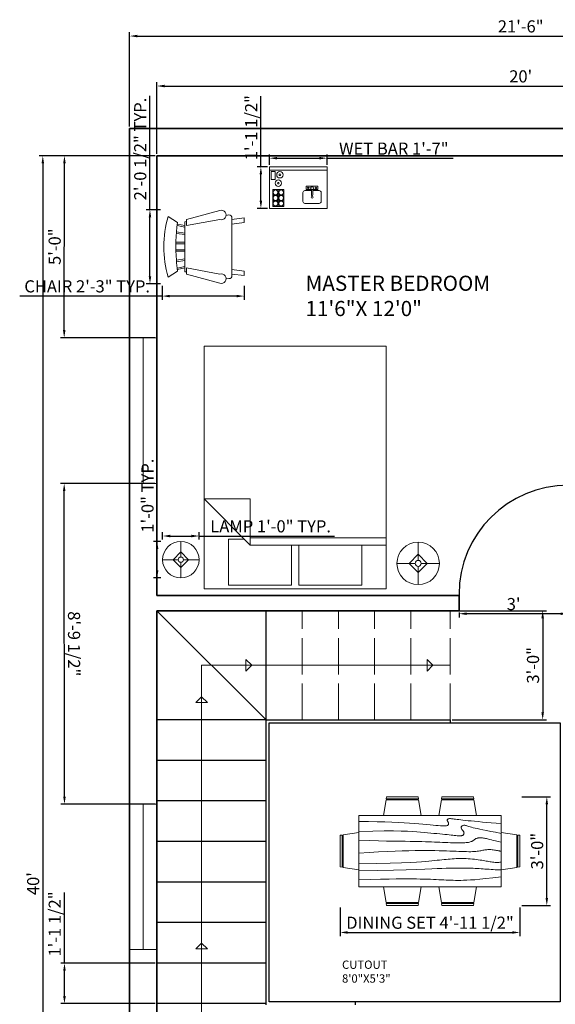
# Model space of a CAD drawing. Units: inches. Extents: x 2170 to 3011, y 1733 to 2338.
# Tile 2 of 5: x 2170 to 2347, y 2014 to 2338. Entities that reach past the tile are written whole.
import ezdxf

# ---------------------------------------------------------------- set-up
doc = ezdxf.new("R2010")
doc.units = ezdxf.units.IN
doc.linetypes.add('ACAD_ISO02W100', pattern=[15, 12, -3])
for name, color, linetype, lineweight in [('A-ANNO-SYMB', 2, 'Continuous', 13), ('A-AREA-IDEN', 4, 'Continuous', 18), ('A-FLOR-FIXT', 20, 'Continuous', 18), ('A-FLOR-OPEN', 7, 'Continuous', 25), ('A-FLOR-STRS-OVHD', 150, 'ACAD_ISO02W100', 18), ('A-WALL', 7, 'Continuous', 35), ('dim', 11, 'Continuous', 18), ('door', 6, 'Continuous', 25), ('furnitures', 20, 'Continuous', 18), ('stairs', 150, 'Continuous', 25), ('window', 3, 'Continuous', 20)]:
    doc.layers.add(name, color=color, linetype=linetype, lineweight=lineweight)
doc.styles.get("Standard").update_dxf_attribs({"font": 'arial.ttf'})
doc.dimstyles.new('ISO-25', dxfattribs={"dimtxt": 4, "dimasz": 2.5, "dimexe": 1.25, "dimexo": 0.625, "dimtad": 1, "dimlunit": 3, "dimtxsty": 'Standard', "dimcen": 2.5, "dimadec": 0, "dimazin": 0, "dimtfac": 1, "dimtmove": 0, "dimatfit": 3, "dimfxl": 1, "dimarcsym": 0})

# ---------------------------------------------------------------- blocks, each defined once
blk = doc.blocks.new('*U3')
for p, q in [((0, 0), (0, -6)), ((-40, 0), (-40, -6))]:
    blk.add_line(p, q)
blk.add_lwpolyline([(0, 0), (0, 40), (-1.75, 40), (-1.75, 0)], close=True)
blk.add_arc((0, 0), 40, 90, 180)
blk = doc.blocks.new('Bed - Queen')
for p, q in [((0, -80.00003), (0, 0)), ((0, 0), (59.99999, 0)), ((59.99999, 0), (59.99999, -80.00003)), ((7.99999, -1.2), (28.79998, -1.2)), ((7.99999, -14.4), (7.99999, -1.2)), ((28.79998, -1.2), (28.79998, -14.4)), ((31.19999, -1.2), (51.99999, -1.2)), ((31.19999, -14.4), (31.19999, -1.2)), ((51.99999, -1.2), (51.99999, -16.4)), ((0, -14.4), (44.8, -14.4)), ((59.99999, -29.6), (44.8, -14.4)), ((44.8, -14.4), (44.8, -29.6)), ((44.8, -16.8), (0, -16.8)), ((51.99999, -16.4), (46.79936, -16.4)), ((44.8, -29.6), (59.99999, -29.6)), ((59.99999, -80.00003), (0, -80.00003))]:
    blk.add_line(p, q)
blk = doc.blocks.new('Chair - Rocking')
for p, q in [((-8, -4.5), (-10, -1.5)), ((8, -4.5), (10, -1.5)), ((-7.5, -4.5), (-7, -7)), ((-6.5, -7), (-7.02225, -4.43)), ((-4.5, -7), (-4.96674, -4.19951)), ((-4, -7), (-4.40532, -4.16272)), ((-1.5, -4.05012), (-1.5, -7)), ((-1, -7), (-1, -4.05012)), ((1, -7), (1, -4.04655)), ((1.5, -4.05012), (1.5, -7)), ((4, -7), (4.40187, -4.18694)), ((4.5, -7), (4.96761, -4.19437)), ((6.5, -7), (7, -4.4057)), ((7.5, -4.5), (7, -7)), ((-9, -7.5), (-12, -18.49999)), ((-7, -7.5), (-9, -7.5)), ((-9, -18.49999), (-7, -7.5)), ((-8.23428, -6.99939), (-8.3093, -7.47958)), ((-8.23041, -7), (8.23915, -7)), ((7, -7.5), (9, -7.5)), ((9, -18.49999), (7, -7.5)), ((8.31071, -7.48854), (8.23449, -7.00073)), ((9, -7.5), (12, -18.49999)), ((-10.36644, -20.64523), (-10.5, -21.49999)), ((-9, -22.49999), (-9.5, -26.49999)), ((0, -22.49999), (-9.5, -22.49999)), ((-8, -26.49999), (-7.5, -22.49999)), ((0, -22.49999), (9.5, -22.49999)), ((8, -26.49999), (7.5, -22.49999)), ((9, -22.49999), (9.5, -26.49999)), ((10.5, -21.49999), (10.3575, -20.58798)), ((-9.5, -26.49999), (-8, -26.49999)), ((9.5, -26.49999), (8, -26.49999))]:
    blk.add_line(p, q)
for centre, radius, start, end in [((0, -34.08333), 34.08333, 72.93847, 107.0615), ((0, -68.25004), 64.25, 93.92211, 97.15267), ((0, -68.25004), 64.25, 82.84733, 93.92211), ((-10.5, -18.99999), 1.58114, 161.5651, 18.43495), ((10.5, -18.99999), 1.58114, 161.5651, 18.43495), ((-9.5, -21.49999), 1, 180, 270), ((9.5, -21.49999), 1, 270, 0)]:
    blk.add_arc(centre, radius, start, end)
blk = doc.blocks.new('Dining Set - 36 x 72 in.')
for p, q in [((-22.2343, 26.00059), (-23.4847, 17.99762)), ((-22.2304, 26), (-5.7608, 26)), ((-22, 27.5), (-22.1562, 26.50042)), ((-5.8416, 26.5), (-22.1534, 26.5)), ((-22, 27.5), (-6, 27.5)), ((-5.8437, 26.49966), (-6, 27.5)), ((-4.5152, 17.99762), (-5.7655, 25.99926)), ((5.7657, 26.00059), (4.5153, 17.99762)), ((5.7696, 26), (22.2392, 26)), ((6, 27.5), (5.8438, 26.50042)), ((22.1584, 26.5), (5.8466, 26.5)), ((6, 27.5), (22, 27.5)), ((22.1563, 26.49966), (22, 27.5)), ((23.4848, 17.99762), (22.2345, 25.99926)), ((36, 18), (-36, 18)), ((-36, 18), (-36, -18)), ((36, -18), (36, 18)), ((-45.5, 8), (-44.5004, 8.15617)), ((-45.5, 8), (-45.5, -8)), ((-44.5, -8.15843), (-44.5, 8.15338)), ((-44.0006, 8.23428), (-35.9976, 9.48474)), ((-44, 8.23041), (-44, -8.23915)), ((44.0006, 8.23428), (35.9976, 9.48474)), ((44, 8.23041), (44, -8.23915)), ((44.5, -8.15843), (44.5, 8.15338)), ((45.5, 8), (44.5005, 8.15617)), ((45.5, 8), (45.5, -8)), ((-44.4997, -8.15631), (-45.5, -8)), ((-35.9976, -9.48476), (-43.9993, -8.2345)), ((35.9976, -9.48476), (43.9993, -8.2345)), ((44.4997, -8.15631), (45.5, -8)), ((-36, -18), (36, -18)), ((-22.2343, -26.0006), (-23.4847, -17.99762)), ((-4.5152, -17.99762), (-5.7655, -25.99928)), ((5.7657, -26.0006), (4.5153, -17.99762)), ((23.4848, -17.99762), (22.2345, -25.99928)), ((-22.2304, -26), (-5.7608, -26)), ((-22, -27.5), (-22.1562, -26.50044)), ((-5.8416, -26.5), (-22.1534, -26.5)), ((-22, -27.5), (-6, -27.5)), ((-5.8437, -26.49967), (-6, -27.5)), ((5.7696, -26), (22.2392, -26)), ((6, -27.5), (5.8438, -26.50044)), ((22.1584, -26.5), (5.8466, -26.5)), ((6, -27.5), (22, -27.5)), ((22.1563, -26.49967), (22, -27.5))]:
    blk.add_line(p, q)
for points in [[(-36, 15), (-31.1772, 14.97754), (-26.8079, 14.91406), (-22.8538, 14.81543), (-19.276, 14.6875), (-16.0362, 14.53613), (-13.0957, 14.36718), (-10.4159, 14.18652), (-7.9583, 14), (-5.6904, 13.81315), (-3.6035, 13.63021), (-1.6954, 13.45508), (0.0365, 13.29166), (1.5945, 13.14388), (2.9811, 13.01562), (4.1988, 12.9108), (5.25, 12.83333), (6.1393, 12.78613), (6.8802, 12.76823), (7.4883, 12.77767), (7.9792, 12.8125), (8.3685, 12.87077), (8.6719, 12.95052), (8.9049, 13.0498), (9.0833, 13.16666), (9.2205, 13.29899), (9.3216, 13.44401), (9.3895, 13.59879), (9.4271, 13.76041), (9.4373, 13.92594), (9.4232, 14.09245), (9.3875, 14.257), (9.3333, 14.41666), (9.2638, 14.56917), (9.1836, 14.71484), (9.0975, 14.85465), (9.0104, 14.98958), (8.9272, 15.1206), (8.8529, 15.2487), (8.7922, 15.37483), (8.75, 15.5), (8.7305, 15.62467), (8.7344, 15.74739), (8.7617, 15.86621), (8.8125, 15.97916), (8.8867, 16.08431), (8.9844, 16.17968), (9.1055, 16.26334), (9.25, 16.33333), (9.4189, 16.38802), (9.6172, 16.42708), (9.8506, 16.45052), (10.125, 16.45833), (10.4463, 16.45052), (10.8203, 16.42708), (11.2529, 16.38802), (11.75, 16.33333), (12.3184, 16.26318), (12.9694, 16.17838), (13.7151, 16.07991), (14.5677, 15.96875), (15.5395, 15.84586), (16.6426, 15.71224), (17.8893, 15.56884), (19.2917, 15.41666), (20.859, 15.25667), (22.5879, 15.08984), (24.4721, 14.91715), (26.5052, 14.73958), (28.6809, 14.5581), (30.9929, 14.3737), (33.4347, 14.18733), (36, 14)], [(-36, 10), (-28.9766, 10.14274), (-23.1725, 10.20442), (-18.4241, 10.19775), (-14.5677, 10.13541), (-11.4399, 10.03011), (-8.877, 9.89453), (-6.7154, 9.74137), (-4.7917, 9.58333), (-2.9698, 9.43082), (-1.2246, 9.28515), (0.4415, 9.14534), (2.026, 9.01041), (3.5266, 8.87939), (4.9408, 8.7513), (6.266, 8.62516), (7.5, 8.5), (8.6411, 8.37549), (9.6914, 8.2539), (10.6538, 8.13818), (11.5312, 8.03125), (12.3267, 7.93603), (13.043, 7.85547), (13.6831, 7.79248), (14.25, 7.75), (14.7471, 7.7303), (15.1797, 7.73307), (15.5537, 7.75732), (15.875, 7.80208), (16.1494, 7.86637), (16.3828, 7.94922), (16.5811, 8.04964), (16.75, 8.16666), (16.8944, 8.29915), (17.0143, 8.44531), (17.1089, 8.60319), (17.1771, 8.77083), (17.218, 8.94629), (17.2305, 9.1276), (17.2137, 9.31282), (17.1667, 9.5), (17.0895, 9.6875), (16.987, 9.875), (16.8649, 10.0625), (16.7292, 10.25), (16.5856, 10.4375), (16.4401, 10.625), (16.2985, 10.8125), (16.1667, 11), (16.05, 11.18733), (15.9518, 11.3737), (15.8752, 11.5581), (15.8229, 11.73958), (15.798, 11.91715), (15.8034, 12.08984), (15.842, 12.25667), (15.9167, 12.41666), (16.0295, 12.56836), (16.1784, 12.70833), (16.3605, 12.83268), (16.5729, 12.9375), (16.8127, 13.01888), (17.0768, 13.07291), (17.3625, 13.0957), (17.6667, 13.08333), (17.9894, 13.03312), (18.3418, 12.94726), (18.7382, 12.82918), (19.1927, 12.68229), (19.7195, 12.51001), (20.3327, 12.31575), (21.0465, 12.10294), (21.875, 11.875), (22.8357, 11.63354), (23.959, 11.37304), (25.2786, 11.08618), (26.8282, 10.76562), (28.6414, 10.40405), (30.752, 9.99414), (33.1936, 9.52856), (36, 9)], [(-36, 5.5), (-30.7157, 5.3348), (-26.069, 5.20963), (-21.9946, 5.11767), (-18.4271, 5.05208), (-15.3009, 5.00602), (-12.5508, 4.97265), (-10.1112, 4.94515), (-7.9167, 4.91666), (-5.909, 4.88167), (-4.0586, 4.83984), (-2.3429, 4.79215), (-0.7396, 4.73958), (0.7739, 4.6831), (2.22, 4.6237), (3.6213, 4.56233), (5, 4.5), (6.373, 4.43782), (7.7344, 4.3776), (9.0723, 4.32129), (10.375, 4.27083), (11.6309, 4.22819), (12.8281, 4.19531), (13.9551, 4.17415), (15, 4.16666), (15.954, 4.17448), (16.819, 4.19791), (17.6001, 4.23698), (18.3021, 4.29166), (18.9299, 4.36198), (19.4883, 4.44791), (19.9823, 4.54948), (20.4167, 4.66666), (20.7969, 4.79899), (21.1302, 4.94401), (21.4245, 5.09879), (21.6875, 5.26041), (21.9271, 5.42594), (22.1511, 5.59245), (22.3672, 5.757), (22.5834, 5.91666), (22.8065, 6.06868), (23.0404, 6.21093), (23.2879, 6.34147), (23.5521, 6.45833), (23.8358, 6.55957), (24.142, 6.64323), (24.4735, 6.70735), (24.8334, 6.75), (25.2235, 6.76969), (25.642, 6.76692), (26.0858, 6.74267), (26.5521, 6.69791), (27.0379, 6.63362), (27.5404, 6.55078), (28.0565, 6.45036), (28.5834, 6.33333), (29.1242, 6.19987), (29.7071, 6.04687), (30.3661, 5.87044), (31.1354, 5.66666), (32.0493, 5.43164), (33.142, 5.16146), (34.4475, 4.85221), (36, 4.5)], [(-36, -1), (-30.7915, -0.6591), (-26.0195, -0.38216), (-21.6519, -0.16284), (-17.6563, 0.00521), (-14.0005, 0.12833), (-10.6523, 0.21289), (-7.5796, 0.26522), (-4.75, 0.29166), (-2.134, 0.29793), (0.2878, 0.28711), (2.5317, 0.26163), (4.6146, 0.22396), (6.5529, 0.17651), (8.3633, 0.12174), (10.0623, 0.06209), (11.6667, 0), (13.1899, -0.06201), (14.6341, -0.1211), (15.9982, -0.17432), (17.2813, -0.21875), (18.4823, -0.25147), (19.6003, -0.26953), (20.6343, -0.27002), (21.5834, -0.25), (22.4481, -0.20768), (23.2357, -0.14584), (23.9549, -0.06836), (24.6146, 0.02083), (25.2235, 0.11784), (25.7904, 0.21875), (26.3241, 0.31966), (26.8334, 0.41666), (27.3265, 0.50618), (27.8099, 0.58593), (28.2894, 0.65397), (28.7709, 0.70833), (29.2601, 0.74707), (29.763, 0.76823), (30.2855, 0.76985), (30.8334, 0.75), (31.4088, 0.70784), (31.9994, 0.64713), (32.589, 0.57275), (33.1615, 0.48958), (33.7008, 0.4025), (34.1908, 0.3164), (34.6153, 0.23616), (34.9584, 0.16666), (35.2099, 0.11165), (35.3848, 0.07031), (35.504, 0.04069), (35.5886, 0.02083), (35.6594, 0.00879), (35.7377, 0.0026), (35.8442, 0.00032), (36, 0)], [(-36, -6.5), (-27.1843, -6.31267), (-20.084, -6.1263), (-14.469, -5.9419), (-10.1094, -5.76042), (-6.7752, -5.58285), (-4.2363, -5.41016), (-2.2629, -5.24333), (-0.625, -5.08334), (0.8708, -4.93099), (2.2715, -4.78646), (3.5872, -4.64974), (4.8281, -4.52084), (6.0046, -4.39974), (7.127, -4.28646), (8.2053, -4.18099), (9.25, -4.08334), (10.2705, -3.99382), (11.2734, -3.91407), (12.2647, -3.84603), (13.25, -3.79167), (14.2354, -3.75293), (15.2266, -3.73177), (16.2295, -3.73015), (17.25, -3.75), (18.2912, -3.79248), (19.3451, -3.85547), (20.4009, -3.93604), (21.4479, -4.03125), (22.4754, -4.13819), (23.4727, -4.25391), (24.4289, -4.37549), (25.3334, -4.5), (26.1785, -4.62492), (26.9694, -4.74935), (27.7145, -4.87281), (28.4219, -4.99479), (29.1, -5.11483), (29.7572, -5.23242), (30.4016, -5.34709), (31.0417, -5.45834), (31.6837, -5.56437), (32.3262, -5.65821), (32.9658, -5.73153), (33.599, -5.77604), (34.2224, -5.78345), (34.8327, -5.74545), (35.4264, -5.65373), (36, -5.5)], [(-36, -10), (-26.4022, -9.81299), (-18.4675, -9.62891), (-11.9839, -9.45069), (-6.7396, -9.28125), (-2.5226, -9.12354), (0.8789, -8.98047), (3.6769, -8.85498), (6.0833, -8.75), (8.2767, -8.66765), (10.3021, -8.60677), (12.1712, -8.56543), (13.8958, -8.54167), (15.4876, -8.53353), (16.9583, -8.53907), (18.3197, -8.55632), (19.5834, -8.58334), (20.7616, -8.61841), (21.8685, -8.66081), (22.9188, -8.71004), (23.9271, -8.76563), (24.9081, -8.82707), (25.8763, -8.89388), (26.8465, -8.96558), (27.8334, -9.04167), (28.8474, -9.12118), (29.8828, -9.20117), (30.93, -9.27824), (31.9792, -9.34896), (33.0205, -9.40991), (34.0443, -9.45768), (35.0407, -9.48885), (36, -9.5)], [(-36, -14.5), (-30.0881, -14.33513), (-25.0332, -14.21224), (-20.7312, -14.12647), (-17.0781, -14.07292), (-13.97, -14.04671), (-11.3027, -14.04297), (-8.9724, -14.05681), (-6.875, -14.08334), (-4.9224, -14.11833), (-3.0905, -14.16016), (-1.3709, -14.20785), (0.2448, -14.26042), (1.7647, -14.3169), (3.1973, -14.3763), (4.5507, -14.43767), (5.8333, -14.5), (7.0554, -14.5621), (8.235, -14.62175), (9.3922, -14.67652), (10.5469, -14.72396), (11.7192, -14.76164), (12.929, -14.78711), (14.1965, -14.79794), (15.5417, -14.79167), (16.9933, -14.76424), (18.6152, -14.70508), (20.4804, -14.60197), (22.6615, -14.44271), (25.2312, -14.21509), (28.2624, -13.9069), (31.8277, -13.50594), (36, -13)]]:
    blk.add_lwpolyline(points)
blk = doc.blocks.new('Wet Bar')
for p, q in [((0, 0), (36, 0)), ((0, -26), (0, 0)), ((36, 0), (36, -26)), ((0, -2), (36, -2)), ((3.5, -3), (1, -3)), ((1, -3), (1, -8)), ((3.5, -8), (3.5, -3)), ((1, -8), (3.5, -8)), ((2, -14.25), (9, -14.25)), ((2, -24.75), (2, -14.25)), ((2, -17.75), (9, -17.75)), ((5.5, -14.25), (5.5, -24.75)), ((9, -14.25), (9, -24.75)), ((26.2, -17.55), (26.2, -14.1284)), ((27.1001, -17.55), (27.1001, -14.1284)), ((9, -21.25), (2, -21.25)), ((36, -26), (0, -26)), ((9, -24.75), (2, -24.75))]:
    blk.add_line(p, q)
for points in [[(26.2, -14.25), (22.95, -14.25), (22.95, -12.2), (26.75, -12.2)], [(26.7487, -12.2), (30.3501, -12.2), (30.3501, -14.25), (27.1001, -14.25)], [(20.95, -21.75), (20.95, -16.05)], [(22.15, -14.85), (26.2, -14.85)], [(27.1001, -14.85), (31.15, -14.85)], [(32.3501, -16.05), (32.3501, -21.75)], [(31.15, -22.95), (22.15, -22.95)]]:
    blk.add_lwpolyline(points)
for centre, radius in [((6.5, -5), 2), ((6.5, -5), 0.5), ((5.5, -10.25), 2), ((5.5, -10.25), 0.5), ((3.75, -16), 1.5), ((3.75, -19.5), 1.5), ((7.25, -16), 1.5), ((7.25, -19.5), 1.5), ((24.25, -13.25), 0.5), ((26.65, -13.35), 0.9), ((26.65, -19.05), 0.6), ((29, -13.25), 0.5), ((3.75, -23), 1.5), ((7.25, -23), 1.5)]:
    blk.add_circle(centre, radius)
for centre, radius, start, end in [((22.2251, -16.125), 1.2772, 93.36646, 176.6335), ((26.65, -17.55), 0.45, 180, 0), ((31.075, -16.125), 1.2772, 3.366461, 86.63354), ((22.2251, -21.675), 1.2772, 183.3665, 266.6335), ((31.075, -21.675), 1.2772, 273.3665, 356.6335)]:
    blk.add_arc(centre, radius, start, end)
blk = doc.blocks.new('Lamp - Table')
for p, q in [((0, 7), (0, 1)), ((-1, 0), (-7, 0)), ((0, 3), (-3, 0)), ((-3, 0), (0, -3)), ((3, 0), (0, 3)), ((0, -3), (3, 0)), ((1, 0), (7, 0)), ((0, -1), (0, -7))]:
    blk.add_line(p, q)
for radius in [7, 1]:
    blk.add_circle((0, 0), radius)
blk = doc.blocks.new('*D22')
at = {"layer": 'Defpoints', "color": 0, "transparency": 16777216}
for p in [(2455.17, 2316.33), (2215.17, 2293.31), (2455.17, 2293.31)]:
    blk.add_point(p, dxfattribs=at)
at = {"layer": 'dim', "color": 0, "lineweight": -2, "transparency": 16777216}
for p, q in [((2215.17, 2293.93), (2215.17, 2317.58)), ((2217.67, 2316.33), (2452.67, 2316.33)), ((2455.17, 2293.93), (2455.17, 2317.58))]:
    blk.add_line(p, q, dxfattribs=at)
at = {"layer": 'dim', "color": 0, "transparency": 16777216}
for points in [[(2217.67, 2316.74), (2217.67, 2315.91), (2215.17, 2316.33)], [(2452.67, 2316.74), (2452.67, 2315.91), (2455.17, 2316.33)]]:
    blk.add_solid(points, dxfattribs=at)
at = {"layer": 'dim', "color": 0, "transparency": 16777216, "insert": (2335.17, 2318.99), "char_height": 4, "attachment_point": 5}
blk.add_mtext("20'", dxfattribs=at)
blk = doc.blocks.new('*D23')
at = {"layer": 'Defpoints', "color": 0, "transparency": 16777216}
for p in [(2215.17, 2293.31), (2177.52, 1813.31), (2215.17, 1813.31)]:
    blk.add_point(p, dxfattribs=at)
at = {"layer": 'dim', "color": 0, "lineweight": -2, "transparency": 16777216}
for p, q in [((2214.54, 2293.31), (2176.27, 2293.31)), ((2177.52, 2290.81), (2177.52, 1815.81)), ((2214.54, 1813.31), (2176.27, 1813.31))]:
    blk.add_line(p, q, dxfattribs=at)
at = {"layer": 'dim', "color": 0, "transparency": 16777216}
for points in [[(2177.11, 2290.81), (2177.94, 2290.81), (2177.52, 2293.31)], [(2177.11, 1815.81), (2177.94, 1815.81), (2177.52, 1813.31)]]:
    blk.add_solid(points, dxfattribs=at)
at = {"layer": 'dim', "color": 0, "transparency": 16777216, "insert": (2174.86, 2053.31), "char_height": 4, "attachment_point": 5, "rotation": 90}
blk.add_mtext("40'", dxfattribs=at)
blk = doc.blocks.new('*D24')
at = {"layer": 'Defpoints', "color": 0, "transparency": 16777216}
for p in [(2314.84, 2143.31), (2350.84, 2143.31), (2314.84, 2142.31)]:
    blk.add_point(p, dxfattribs=at)
at = {"layer": 'dim', "color": 0, "lineweight": -2, "transparency": 16777216}
for p, q in [((2314.84, 2142.68), (2314.84, 2141.06)), ((2348.34, 2142.31), (2317.34, 2142.31)), ((2350.84, 2142.68), (2350.84, 2141.06))]:
    blk.add_line(p, q, dxfattribs=at)
at = {"layer": 'dim', "color": 0, "transparency": 16777216}
for points in [[(2317.34, 2142.73), (2317.34, 2141.9), (2314.84, 2142.31)], [(2348.34, 2142.73), (2348.34, 2141.9), (2350.84, 2142.31)]]:
    blk.add_solid(points, dxfattribs=at)
at = {"layer": 'dim', "color": 0, "transparency": 16777216, "insert": (2332.84, 2144.98), "char_height": 4, "attachment_point": 5}
blk.add_mtext("3'", dxfattribs=at)
blk = doc.blocks.new('WINDOW-48x9')
blk.add_line((4.5, 48), (4.5, 0))
blk.add_lwpolyline([(0, 48), (9, 48), (9, 0), (0, 0)], close=True)
blk = doc.blocks.new('STAIR-UP-PATH')
for p, q in [((16.56, 133.24), (16.56, 137.12)), ((16.56, 137.12), (18.45, 135.18)), ((76.31, 133.24), (76.31, 137.12)), ((76.31, 137.12), (78.21, 135.18)), ((1.94, 1.94), (1.94, 135.18)), ((1.94, 135.18), (83.94, 135.18)), ((16.56, 133.24), (18.45, 135.18)), ((76.31, 133.24), (78.21, 135.18)), ((0, 122.86), (1.94, 124.75)), ((3.88, 122.86), (1.94, 124.75)), ((3.88, 122.86), (0, 122.86)), ((0, 41.63), (1.94, 43.52)), ((3.88, 41.63), (1.94, 43.52)), ((3.88, 41.63), (0, 41.63)), ((9.93, 3.88), (8.04, 1.94)), ((9.93, 3.88), (9.93, 0)), ((50.68, 3.88), (48.79, 1.94)), ((50.68, 3.88), (50.68, 0)), ((55.9, 1.94), (1.94, 1.94)), ((9.93, 0), (8.04, 1.94)), ((50.68, 0), (48.79, 1.94))]:
    blk.add_line(p, q)
blk = doc.blocks.new('*D46')
at = {"layer": 'Defpoints', "color": 0, "transparency": 16777216}
for p in [(2216.92, 2251.11), (2243.92, 2251.11), (2216.92, 2247.06)]:
    blk.add_point(p, dxfattribs=at)
at = {"layer": 'dim', "color": 0, "lineweight": -2, "transparency": 16777216}
for p, q in [((2216.92, 2250.48), (2216.92, 2245.81)), ((2243.92, 2250.48), (2243.92, 2245.81)), ((2216.92, 2247.06), (2169.9, 2247.06)), ((2241.42, 2247.06), (2219.42, 2247.06))]:
    blk.add_line(p, q, dxfattribs=at)
at = {"layer": 'dim', "color": 0, "transparency": 16777216}
for points in [[(2219.42, 2247.48), (2219.42, 2246.64), (2216.92, 2247.06)], [(2241.42, 2247.48), (2241.42, 2246.64), (2243.92, 2247.06)]]:
    blk.add_solid(points, dxfattribs=at)
at = {"layer": 'dim', "color": 0, "transparency": 16777216, "insert": (2192.16, 2249.75), "char_height": 4, "attachment_point": 5}
blk.add_mtext('CHAIR 2\'-3" TYP.', dxfattribs=at)
blk = doc.blocks.new('*D47')
at = {"layer": 'Defpoints', "color": 0, "transparency": 16777216}
for p in [(2212.87, 2275.55), (2216.92, 2275.55), (2216.92, 2251.11)]:
    blk.add_point(p, dxfattribs=at)
at = {"layer": 'dim', "color": 0, "lineweight": -2, "transparency": 16777216}
for p, q in [((2212.87, 2275.55), (2212.87, 2313.07)), ((2216.3, 2275.55), (2211.62, 2275.55)), ((2212.87, 2253.61), (2212.87, 2273.05)), ((2216.3, 2251.11), (2211.62, 2251.11))]:
    blk.add_line(p, q, dxfattribs=at)
at = {"layer": 'dim', "color": 0, "transparency": 16777216}
for points in [[(2212.46, 2273.05), (2213.29, 2273.05), (2212.87, 2275.55)], [(2212.46, 2253.61), (2213.29, 2253.61), (2212.87, 2251.11)]]:
    blk.add_solid(points, dxfattribs=at)
at = {"layer": 'dim', "color": 0, "transparency": 16777216, "insert": (2210.18, 2295.56), "char_height": 4, "attachment_point": 5, "rotation": 90}
blk.add_mtext('2\'-0 1/2" TYP.', dxfattribs=at)
blk = doc.blocks.new('*D48')
at = {"layer": 'Defpoints', "color": 0, "transparency": 16777216}
for p in [(2217.05, 2166.14), (2229.07, 2167.94), (2229.07, 2166.14)]:
    blk.add_point(p, dxfattribs=at)
at = {"layer": 'dim', "color": 0, "lineweight": -2, "transparency": 16777216}
for p, q in [((2217.05, 2166.76), (2217.05, 2169.19)), ((2229.07, 2166.76), (2229.07, 2169.19)), ((2219.55, 2167.94), (2226.57, 2167.94)), ((2229.07, 2167.94), (2273.79, 2167.94))]:
    blk.add_line(p, q, dxfattribs=at)
at = {"layer": 'dim', "color": 0, "transparency": 16777216}
for points in [[(2219.55, 2168.35), (2219.55, 2167.52), (2217.05, 2167.94)], [(2226.57, 2168.35), (2226.57, 2167.52), (2229.07, 2167.94)]]:
    blk.add_solid(points, dxfattribs=at)
at = {"layer": 'dim', "color": 0, "transparency": 16777216, "insert": (2252.68, 2170.61), "char_height": 4, "attachment_point": 5}
blk.add_mtext('LAMP 1\'-0" TYP.', dxfattribs=at)
blk = doc.blocks.new('*D49')
at = {"layer": 'Defpoints', "color": 0, "transparency": 16777216}
for p in [(2215.24, 2166.14), (2217.05, 2166.14), (2217.05, 2154.12)]:
    blk.add_point(p, dxfattribs=at)
at = {"layer": 'dim', "color": 0, "lineweight": -2, "transparency": 16777216}
for p, q in [((2215.24, 2166.14), (2215.24, 2193.89)), ((2216.42, 2166.14), (2213.99, 2166.14)), ((2215.24, 2156.62), (2215.24, 2163.64)), ((2216.42, 2154.12), (2213.99, 2154.12))]:
    blk.add_line(p, q, dxfattribs=at)
at = {"layer": 'dim', "color": 0, "transparency": 16777216}
for points in [[(2214.83, 2163.64), (2215.66, 2163.64), (2215.24, 2166.14)], [(2214.83, 2156.62), (2215.66, 2156.62), (2215.24, 2154.12)]]:
    blk.add_solid(points, dxfattribs=at)
at = {"layer": 'dim', "color": 0, "transparency": 16777216, "insert": (2212.58, 2181.26), "char_height": 4, "attachment_point": 5, "rotation": 90}
blk.add_mtext('1\'-0" TYP.', dxfattribs=at)
blk = doc.blocks.new('*D74')
at = {"layer": 'Defpoints', "color": 0, "transparency": 16777216}
for p in [(2275.59, 2046.1), (2334.89, 2046.1), (2334.89, 2037.21)]:
    blk.add_point(p, dxfattribs=at)
at = {"layer": 'dim', "color": 0, "lineweight": -2, "transparency": 16777216}
for p, q in [((2275.59, 2045.48), (2275.59, 2035.96)), ((2334.89, 2045.48), (2334.89, 2035.96)), ((2278.09, 2037.21), (2332.39, 2037.21))]:
    blk.add_line(p, q, dxfattribs=at)
at = {"layer": 'dim', "color": 0, "transparency": 16777216}
for points in [[(2278.09, 2037.63), (2278.09, 2036.79), (2275.59, 2037.21)], [(2332.39, 2037.63), (2332.39, 2036.79), (2334.89, 2037.21)]]:
    blk.add_solid(points, dxfattribs=at)
at = {"layer": 'dim', "color": 0, "transparency": 16777216, "insert": (2305.24, 2039.9), "char_height": 4, "attachment_point": 5}
blk.add_mtext('DINING SET 4\'-11 1/2"', dxfattribs=at)
blk = doc.blocks.new('*D75')
at = {"layer": 'Defpoints', "color": 0, "transparency": 16777216}
for p in [(2334.89, 2081.95), (2343.79, 2081.95), (2334.89, 2046.1)]:
    blk.add_point(p, dxfattribs=at)
at = {"layer": 'dim', "color": 0, "lineweight": -2, "transparency": 16777216}
for p, q in [((2335.52, 2081.95), (2345.04, 2081.95)), ((2343.79, 2048.6), (2343.79, 2079.45)), ((2335.52, 2046.1), (2345.04, 2046.1))]:
    blk.add_line(p, q, dxfattribs=at)
at = {"layer": 'dim', "color": 0, "transparency": 16777216}
for points in [[(2343.37, 2079.45), (2344.2, 2079.45), (2343.79, 2081.95)], [(2343.37, 2048.6), (2344.2, 2048.6), (2343.79, 2046.1)]]:
    blk.add_solid(points, dxfattribs=at)
at = {"layer": 'dim', "color": 0, "transparency": 16777216, "insert": (2341.12, 2064.03), "char_height": 4, "attachment_point": 5, "rotation": 90}
blk.add_mtext('3\'-0"', dxfattribs=at)
blk = doc.blocks.new('*D76')
at = {"layer": 'Defpoints', "color": 0, "transparency": 16777216}
for p in [(2271.28, 2292.53), (2252.31, 2289.69), (2271.28, 2289.69)]:
    blk.add_point(p, dxfattribs=at)
at = {"layer": 'dim', "color": 0, "lineweight": -2, "transparency": 16777216}
for p, q in [((2252.31, 2290.31), (2252.31, 2293.78)), ((2254.81, 2292.53), (2268.78, 2292.53)), ((2271.28, 2290.31), (2271.28, 2293.78)), ((2271.28, 2292.53), (2312.84, 2292.53))]:
    blk.add_line(p, q, dxfattribs=at)
at = {"layer": 'dim', "color": 0, "transparency": 16777216}
for points in [[(2254.81, 2292.95), (2254.81, 2292.12), (2252.31, 2292.53)], [(2268.78, 2292.95), (2268.78, 2292.12), (2271.28, 2292.53)]]:
    blk.add_solid(points, dxfattribs=at)
at = {"layer": 'dim', "color": 0, "transparency": 16777216, "insert": (2293.31, 2295.17), "char_height": 4, "attachment_point": 5}
blk.add_mtext('WET BAR 1\'-7"', dxfattribs=at)
blk = doc.blocks.new('*D77')
at = {"layer": 'Defpoints', "color": 0, "transparency": 16777216}
for p in [(2249.46, 2289.69), (2252.31, 2289.69), (2252.31, 2275.99)]:
    blk.add_point(p, dxfattribs=at)
at = {"layer": 'dim', "color": 0, "lineweight": -2, "transparency": 16777216}
for p, q in [((2249.46, 2289.69), (2249.46, 2313.02)), ((2251.68, 2289.69), (2248.21, 2289.69)), ((2249.46, 2278.49), (2249.46, 2287.19)), ((2251.68, 2275.99), (2248.21, 2275.99))]:
    blk.add_line(p, q, dxfattribs=at)
at = {"layer": 'dim', "color": 0, "transparency": 16777216}
for points in [[(2249.04, 2287.19), (2249.88, 2287.19), (2249.46, 2289.69)], [(2249.04, 2278.49), (2249.88, 2278.49), (2249.46, 2275.99)]]:
    blk.add_solid(points, dxfattribs=at)
at = {"layer": 'dim', "color": 0, "transparency": 16777216, "insert": (2246.77, 2302.6), "char_height": 4, "attachment_point": 5, "rotation": 90}
blk.add_mtext('1\'-1 1/2"', dxfattribs=at)
blk = doc.blocks.new('*D83')
at = {"layer": 'Defpoints', "color": 0, "transparency": 16777216}
for p in [(2184.67, 2293.35), (2215.17, 2293.31), (2215.08, 2233.28)]:
    blk.add_point(p, dxfattribs=at)
at = {"layer": 'dim', "color": 0, "lineweight": -2, "transparency": 16777216}
for p, q in [((2214.54, 2293.31), (2183.42, 2293.35)), ((2184.59, 2235.82), (2184.67, 2290.85)), ((2214.46, 2233.28), (2183.33, 2233.32))]:
    blk.add_line(p, q, dxfattribs=at)
at = {"layer": 'dim', "color": 0, "transparency": 16777216}
for points in [[(2184.25, 2290.85), (2185.08, 2290.85), (2184.67, 2293.35)], [(2184.17, 2235.82), (2185, 2235.82), (2184.58, 2233.32)]]:
    blk.add_solid(points, dxfattribs=at)
at = {"layer": 'dim', "color": 0, "transparency": 16777216, "insert": (2181.96, 2263.34), "char_height": 4, "attachment_point": 5, "rotation": 89.9191}
blk.add_mtext('5\'-0"', dxfattribs=at)
blk = doc.blocks.new('*D84')
at = {"layer": 'Defpoints', "color": 0, "transparency": 16777216}
for p in [(2184.58, 2185.25), (2215.08, 2185.28), (2215.17, 2079.54)]:
    blk.add_point(p, dxfattribs=at)
at = {"layer": 'dim', "color": 0, "lineweight": -2, "transparency": 16777216}
for p, q in [((2214.46, 2185.28), (2183.33, 2185.25)), ((2184.67, 2082.02), (2184.59, 2182.75)), ((2214.54, 2079.54), (2183.42, 2079.52))]:
    blk.add_line(p, q, dxfattribs=at)
at = {"layer": 'dim', "color": 0, "transparency": 16777216}
for points in [[(2185, 2182.75), (2184.17, 2182.75), (2184.58, 2185.25)], [(2185.08, 2082.02), (2184.25, 2082.02), (2184.67, 2079.52)]]:
    blk.add_solid(points, dxfattribs=at)
at = {"layer": 'dim', "color": 0, "transparency": 16777216, "insert": (2187.32, 2132.39), "char_height": 4, "attachment_point": 5, "rotation": 270.046}
blk.add_mtext('8\'-9 1/2"', dxfattribs=at)
blk = doc.blocks.new('*D88')
at = {"layer": 'Defpoints', "color": 0, "transparency": 16777216}
for p in [(2311.92, 2143.31), (2311.92, 2107.31), (2342.42, 2107.31)]:
    blk.add_point(p, dxfattribs=at)
at = {"layer": 'dim', "color": 0, "lineweight": -2, "transparency": 16777216}
for p, q in [((2312.55, 2143.31), (2343.67, 2143.31)), ((2342.42, 2140.81), (2342.42, 2109.81)), ((2312.55, 2107.31), (2343.67, 2107.31))]:
    blk.add_line(p, q, dxfattribs=at)
at = {"layer": 'dim', "color": 0, "transparency": 16777216}
for points in [[(2342, 2140.81), (2342.84, 2140.81), (2342.42, 2143.31)], [(2342, 2109.81), (2342.84, 2109.81), (2342.42, 2107.31)]]:
    blk.add_solid(points, dxfattribs=at)
at = {"layer": 'dim', "color": 0, "transparency": 16777216, "insert": (2339.75, 2125.31), "char_height": 4, "attachment_point": 5, "rotation": 90}
blk.add_mtext('3\'-0"', dxfattribs=at)
blk = doc.blocks.new('*D89')
at = {"layer": 'Defpoints', "color": 0, "transparency": 16777216}
for p in [(2184.67, 2027.1), (2215.17, 2027.1), (2215.17, 2013.73)]:
    blk.add_point(p, dxfattribs=at)
at = {"layer": 'dim', "color": 0, "lineweight": -2, "transparency": 16777216}
for p, q in [((2184.67, 2027.1), (2184.67, 2050.43)), ((2214.54, 2027.1), (2183.42, 2027.1)), ((2184.67, 2016.23), (2184.67, 2024.6)), ((2214.54, 2013.73), (2183.42, 2013.73))]:
    blk.add_line(p, q, dxfattribs=at)
at = {"layer": 'dim', "color": 0, "transparency": 16777216}
for points in [[(2184.25, 2024.6), (2185.09, 2024.6), (2184.67, 2027.1)], [(2184.25, 2016.23), (2185.09, 2016.23), (2184.67, 2013.73)]]:
    blk.add_solid(points, dxfattribs=at)
at = {"layer": 'dim', "color": 0, "transparency": 16777216, "insert": (2181.98, 2040.01), "char_height": 4, "attachment_point": 5, "rotation": 90}
blk.add_mtext('1\'-1 1/2"', dxfattribs=at)
blk = doc.blocks.new('*D100')
at = {"layer": 'Defpoints', "color": 0, "transparency": 16777216}
for p in [(2464.17, 2332.81), (2206.17, 2302.31), (2464.17, 2302.31)]:
    blk.add_point(p, dxfattribs=at)
at = {"layer": 'dim', "color": 0, "lineweight": -2, "transparency": 16777216}
for p, q in [((2206.17, 2302.93), (2206.17, 2334.06)), ((2208.67, 2332.81), (2461.67, 2332.81)), ((2464.17, 2302.93), (2464.17, 2334.06))]:
    blk.add_line(p, q, dxfattribs=at)
at = {"layer": 'dim', "color": 0, "transparency": 16777216}
for points in [[(2208.67, 2333.22), (2208.67, 2332.39), (2206.17, 2332.81)], [(2461.67, 2333.22), (2461.67, 2332.39), (2464.17, 2332.81)]]:
    blk.add_solid(points, dxfattribs=at)
at = {"layer": 'dim', "color": 0, "transparency": 16777216, "insert": (2335.17, 2335.47), "char_height": 4, "attachment_point": 5}
blk.add_mtext('21\'-6"', dxfattribs=at)

msp = doc.modelspace()

# ---------------------------------------------------------------- linework, layer by layer
at = {"layer": 'A-FLOR-OPEN'}
msp.add_lwpolyline([(2252.169, 2106.306), (2348.169, 2106.306), (2348.169, 2014.306), (2252.169, 2014.306)], close=True, dxfattribs=at)
at = {"layer": 'A-FLOR-STRS-OVHD'}
for p, q in [((2263.104, 2107.306), (2263.104, 2143.306)), ((2275.039, 2107.306), (2275.039, 2143.306)), ((2286.975, 2107.306), (2286.975, 2143.306)), ((2298.91, 2107.306), (2298.91, 2143.306)), ((2311.921, 2107.306), (2311.921, 2143.306))]:
    msp.add_line(p, q, dxfattribs=at)
at = {"layer": 'A-WALL'}
for p, q in [((2206.169, 1804.306), (2206.169, 2302.306)), ((2206.169, 2302.306), (2464.169, 2302.306)), ((2215.169, 2293.306), (2455.169, 2293.306)), ((2215.169, 2148.306), (2215.169, 2293.306)), ((2215.169, 2148.306), (2314.84, 2148.306)), ((2215.169, 2143.306), (2314.84, 2143.306)), ((2215.169, 1977.306), (2215.169, 2143.306))]:
    msp.add_line(p, q, dxfattribs=at)
msp.add_lwpolyline([(2314.84, 2143.306), (2314.84, 2148.306)], dxfattribs=at)
at = {"layer": 'door'}
msp.add_lwpolyline([(2314.84, 2143.306), (2314.84, 2148.306)], dxfattribs=at)
at = {"layer": 'stairs'}
for p, q in [((2251.169, 2107.306), (2215.169, 2143.306)), ((2251.169, 2107.306), (2251.169, 2143.306)), ((2251.169, 2107.306), (2215.169, 2107.306)), ((2251.169, 2013.306), (2251.169, 2107.306)), ((2251.169, 2107.306), (2287.512, 2107.306)), ((2287.512, 2107.306), (2311.921, 2107.306)), ((2311.921, 2107.306), (2311.921, 2106.306)), ((2252.169, 2106.306), (2287.512, 2106.306)), ((2252.169, 2014.306), (2252.169, 2106.306)), ((2287.512, 2106.306), (2311.921, 2106.306)), ((2251.169, 2093.938), (2215.169, 2093.938)), ((2251.169, 2080.57), (2215.169, 2080.57)), ((2251.169, 2067.202), (2215.169, 2067.202)), ((2251.169, 2053.834), (2215.169, 2053.834)), ((2251.169, 2040.466), (2215.169, 2040.466)), ((2251.169, 2027.098), (2215.169, 2027.098)), ((2251.169, 2013.73), (2215.169, 2013.73)), ((2280.513, 2014.306), (2252.169, 2014.306)), ((2280.513, 2014.306), (2280.513, 2013.306))]:
    msp.add_line(p, q, dxfattribs=at)

# ---------------------------------------------------------------- block references
at = {"layer": 'A-ANNO-SYMB'}
msp.add_blockref('STAIR-UP-PATH', (2227.984, 1990.129), dxfattribs=at)
at = {"layer": 'A-FLOR-FIXT', "xscale": 0.5270462766947299, "yscale": 0.5270462766947299, "zscale": 0.5270462766947299}
msp.add_blockref('Wet Bar', (2252.306, 2289.688), dxfattribs=at)
at = {"layer": 'door', "xscale": 0.9, "yscale": 0.9, "zscale": 0.9}
msp.add_blockref('*U3', (2350.84, 2148.706), dxfattribs=at)
at = {"layer": 'furnitures'}
for name, p, rotation in [('Chair - Rocking', (2217.423, 2263.327), 90), ('Bed - Queen', (2290.767, 2150.548), 180)]:
    msp.add_blockref(name, p, dxfattribs=dict(at, rotation=rotation))
for name, p, xscale, yscale, zscale in [('Lamp - Table', (2223.058, 2160.125), 0.8585674405306916, 0.8585674405306916, 0.8585674405306916), ('Dining Set - 36 x 72 in.', (2305.242, 2064.026), 0.6516612372804925, 0.6516612372804925, 0.6516612372804925)]:
    msp.add_blockref(name, p, dxfattribs=dict(at, xscale=xscale, yscale=yscale, zscale=zscale))
msp.add_blockref('Lamp - Table', (2301.352, 2158.909), dxfattribs=at)
at = {"layer": 'window'}
for p in [(2206.084, 2185.278), (2206.169, 2031.545)]:
    msp.add_blockref('WINDOW-48x9', p, dxfattribs=at)

# ---------------------------------------------------------------- texts
at = {"layer": 'A-AREA-IDEN', "attachment_point": 1}
for s, width, gutter_width, insert, char_height in [('MASTER BEDROOM\\P11\'6"X 12\'0"', 81.99853, 12.5, (2264.189, 2253.788), 5), ('CUTOUT\\P8\'0"X5\'3"', 27.0623, 6.833, (2276.233, 2027.948), 2.7333)]:
    msp.add_mtext_dynamic_manual_height_columns(s, width=width, gutter_width=gutter_width, heights=[0], dxfattribs=dict(at, insert=insert, char_height=char_height))

# ---------------------------------------------------------------- dimensions: what is measured, and where the dimension line sits
at = {"layer": 'dim'}
for base, p1, p2, override, picture, middle in [((2464.169, 2332.806), (2206.169, 2302.306), (2464.169, 2302.306), {"dimdec": 1, "dimlfac": 1, "dimrnd": 0, "dimzin": 1, "dimdsep": 46, "dimlunit": 4, "dimfrac": 2}, '*D100', (2335.169, 2335.474)), ((2455.169, 2316.325), (2215.169, 2293.306), (2455.169, 2293.306), {"dimclrd": 0, "dimclre": 0, "dimclrt": 0}, '*D22', (2335.169, 2318.992)), ((2314.84, 2142.315), (2350.84, 2143.306), (2314.84, 2143.306), {"dimclrd": 0, "dimclre": 0, "dimclrt": 0}, '*D24', (2332.84, 2144.984))]:
    dim = msp.add_linear_dim(base=base, p1=p1, p2=p2, dimstyle='ISO-25', override=override, dxfattribs=at)
    dim.commit()
    dim.dimension.update_dxf_attribs({"geometry": picture, "text_midpoint": middle})
for base, p1, p2, angle, text, picture, middle in [((2212.873, 2275.545), (2216.923, 2251.11), (2216.923, 2275.545), 90, '<> TYP.', '*D47', (2210.18, 2295.555)), ((2216.923, 2247.06), (2243.923, 2251.11), (2216.923, 2251.11), 180, 'CHAIR <> TYP.', '*D46', (2192.161, 2249.755)), ((2215.245, 2166.135), (2217.048, 2154.115), (2217.048, 2166.135), 90, '<> TYP.', '*D49', (2212.577, 2181.263))]:
    dim = msp.add_linear_dim(base=base, p1=p1, p2=p2, angle=angle, text=text, dimstyle='ISO-25', override={"dimdec": 1, "dimlfac": 1, "dimrnd": 0, "dimzin": 1, "dimdsep": 46, "dimlunit": 4, "dimfrac": 2}, dxfattribs=at)
    dim.commit()
    dim.dimension.update_dxf_attribs({"geometry": picture, "text_midpoint": middle})
for base, p1, p2, angle, override, picture, middle in [((2249.46, 2289.688), (2252.306, 2275.985), (2252.306, 2289.688), 90, {"dimdec": 1, "dimlfac": 1, "dimrnd": 0, "dimzin": 1, "dimdsep": 46, "dimlunit": 4, "dimfrac": 2}, '*D77', (2246.767, 2302.602)), ((2177.525, 1813.306), (2215.169, 2293.306), (2215.169, 1813.306), 90, {"dimclrd": 0, "dimclre": 0, "dimclrt": 0}, '*D23', (2174.857, 2053.306)), ((2184.669, 2293.349), (2215.084, 2233.278), (2215.169, 2293.306), 89.91906, {"dimdec": 1, "dimlfac": 1, "dimrnd": 0, "dimzin": 1, "dimdsep": 46, "dimlunit": 4, "dimfrac": 2}, '*D83', (2181.96, 2263.339)), ((2184.584, 2185.253), (2215.169, 2079.545), (2215.084, 2185.278), 90.04596, {"dimdec": 1, "dimlfac": 1, "dimrnd": 0, "dimzin": 1, "dimdsep": 46, "dimlunit": 4, "dimfrac": 2}, '*D84', (2187.32, 2132.389)), ((2342.421, 2107.306), (2311.921, 2143.306), (2311.921, 2107.306), 270, {"dimdec": 1, "dimlfac": 1, "dimrnd": 0, "dimzin": 1, "dimdsep": 46, "dimlunit": 4, "dimfrac": 2}, '*D88', (2339.753, 2125.306)), ((2343.788, 2081.946), (2334.893, 2046.105), (2334.893, 2081.946), 90, {"dimdec": 1, "dimlfac": 1, "dimrnd": 0, "dimzin": 1, "dimdsep": 46, "dimlunit": 4, "dimfrac": 2}, '*D75', (2341.119, 2064.026)), ((2184.669, 2027.098), (2215.169, 2013.73), (2215.169, 2027.098), 90, {"dimdec": 1, "dimlfac": 1, "dimrnd": 0, "dimzin": 1, "dimdsep": 46, "dimlunit": 4, "dimfrac": 2}, '*D89', (2181.976, 2040.012))]:
    dim = msp.add_linear_dim(base=base, p1=p1, p2=p2, angle=angle, dimstyle='ISO-25', override=override, dxfattribs=at)
    dim.commit()
    dim.dimension.update_dxf_attribs({"geometry": picture, "text_midpoint": middle})
for base, p1, p2, text, picture, middle in [((2271.28, 2292.534), (2252.306, 2289.688), (2271.28, 2289.688), 'WET BAR <>', '*D76', (2293.308, 2295.169)), ((2229.068, 2167.938), (2217.048, 2166.135), (2229.068, 2166.135), 'LAMP <> TYP.', '*D48', (2252.68, 2170.605)), ((2334.893, 2037.21), (2275.591, 2046.105), (2334.893, 2046.105), 'DINING SET <>', '*D74', (2305.242, 2039.903))]:
    dim = msp.add_linear_dim(base=base, p1=p1, p2=p2, text=text, dimstyle='ISO-25', override={"dimdec": 1, "dimlfac": 1, "dimrnd": 0, "dimzin": 1, "dimdsep": 46, "dimlunit": 4, "dimfrac": 2}, dxfattribs=at)
    dim.commit()
    dim.dimension.update_dxf_attribs({"geometry": picture, "text_midpoint": middle})

doc.saveas('drawing.dxf')
